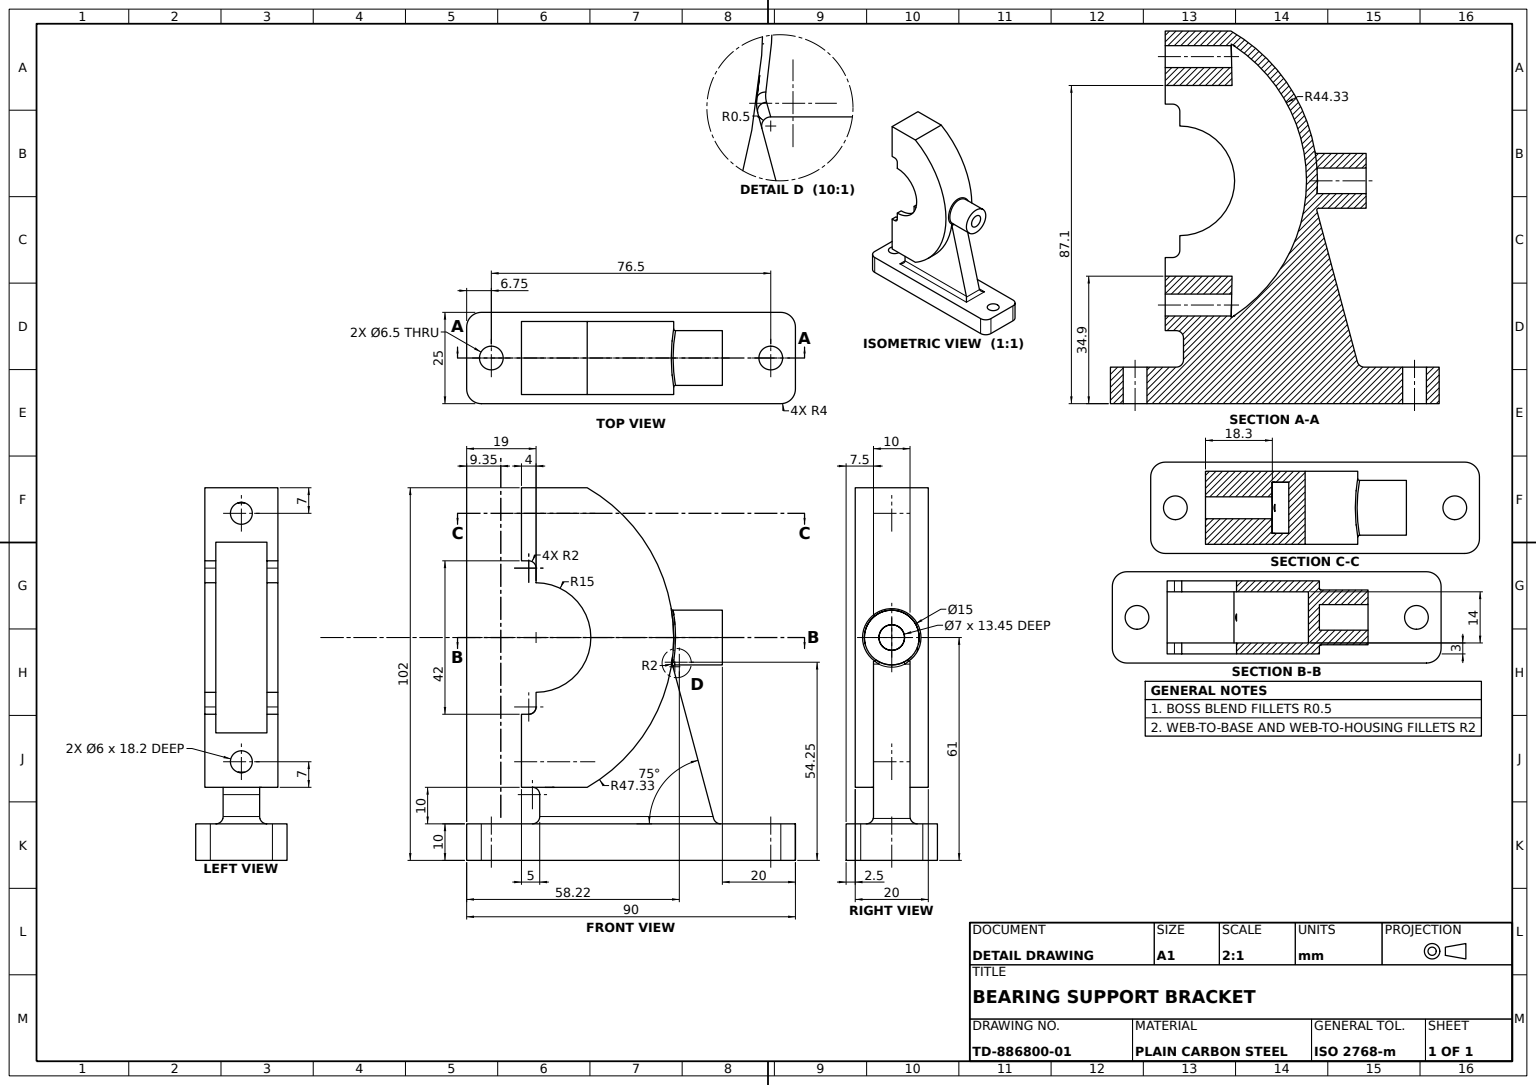
SolidWorks part; units mm, degrees
material "Plain Carbon Steel"
ref_plane "Front Plane" through (0, 0, 0) normal (0, 0, 1) x (1, 0, 0)
ref_plane "Top Plane" through (0, 0, 0) normal (0, 1, 0) x (1, 0, 0)
ref_plane "Right Plane" through (0, 0, 0) normal (1, 0, 0) x (0, 0, -1)
sketch "Base Plate Sketch" plane through (0, 0, 0) normal (0, 1, 0) x (1, 0, 0)
  line L1 (-41, 12.5) -> (41, 12.5)
  line L2 (-45, 8.5) -> (-45, -8.5)
  line L3 (-41, -12.5) -> (41, -12.5)
  line L4 (45, 8.5) -> (45, -8.5)
  line L5 (-45, 12.5) -> (45, -12.5) construction
  line L6 (-45, -12.5) -> (45, 12.5) construction
  arc A0 (41, -12.5) -> (45, -8.5) centre (41, -8.5) ccw
  arc A1 (41, 12.5) -> (45, 8.5) centre (41, 8.5) cw
  arc A2 (-45, -8.5) -> (-41, -12.5) centre (-41, -8.5) ccw
  arc A3 (-41, 12.5) -> (-45, 8.5) centre (-41, 8.5) ccw
  point P0 (0, 0)
  dimension "D3" = 4
  dimension "D1" = 90
  dimension "D2" = 25
extrude "Base Plate" add sketch "Base Plate Sketch" along normal blind 10
sketch "Mounting Holes Sketch" plane through (0, 10, 0) normal (0, 1, 0) x (1, 0, 0)
  line L0 (45, -8.5) -> (45, 8.5) construction
  line L1 (41, 12.5) -> (-41, 12.5) construction
  line L3 (-45, 8.5) -> (-45, -8.5) construction
  circle A0 centre (-38.25, 0) radius 3.25
  circle A1 centre (38.25, 0) radius 3.25
  dimension "D1" = 6.5
  dimension "D2" = 6.5
  dimension "D3" = 76.5
  dimension "D4" = 6.75
  dimension "D5" = 12.5
  dimension "D6" = 6.75
extrude "Mounting Holes 2xØ6.5" cut sketch "Mounting Holes Sketch" against normal blind 10
sketch "Upright Web Sketch" plane through (0, 10, 0) normal (0, 1, 0) x (1, 0, 0)
  line L1 (-24, 6) -> (24, 6)
  line L2 (-24, 6) -> (-24, -6)
  line L3 (-24, -6) -> (24, -6)
  line L4 (24, 6) -> (24, -6)
  line L5 (-24, 6) -> (24, -6) construction
  line L6 (-24, -6) -> (24, 6) construction
  point P0 (0, 0)
  dimension "D1" = 12
  dimension "D2" = 48
extrude "Upright Web" add sketch "Upright Web Sketch" along normal blind 30 draft 3
ref_plane "Plane1" through (0, 0, 10) normal (0, 0, 1) x (1, 0, 0)
sketch "Housing Half Sketch" plane through (0, 0, 10) normal (0, 0, 1) x (1, 0, 0)
  line L3 (-30, 82) -> (-26, 82)
  line L4 (-30, 102) -> (-12, 102)
  line L5 (-30, 102) -> (-12, 102)
  line L6 (-30, 20) -> (-12, 20)
  line L7 (-30, 40) -> (-30, 20)
  line L8 (-26, 82) -> (-26, 76)
  line L9 (-30, 102) -> (-30, 82)
  line L10 (-30, 40) -> (-26, 40)
  line L11 (-26, 40) -> (-26, 46)
  arc A0 (-12, 102) -> (-12, 20) centre (-35.6548, 61) cw
  arc A1 (-26, 76) -> (-26, 46) centre (-26, 61) cw
  dimension "D3" = 18
  dimension "D6" = 47.3344
  dimension "D14" = 15
  dimension "D1" = 82
  dimension "D2" = 20
  dimension "D4" = 18
  dimension "D5" = 102
  dimension "D7" = 4
  dimension "D8" = 6
  dimension "D9" = 20
  dimension "D10" = 4
  dimension "D11" = 6
  dimension "D12" = 48.4278
  dimension "D13" = 12
extrude "Housing Half" add sketch "Housing Half Sketch" against normal blind 3 separate body contours L8 A1 L11 L10 L7 L6 A0 L4 L9 L3
sketch "Housing Arc Cut Sketch" plane through (0, 0, 7) normal (0, 0, -1) x (-1, 0, 0)
  line L0 (12, 20) -> (30, 20)
  line L1 (30, 20) -> (30, 40)
  line L2 (30, 40) -> (-6.7663, 40)
  line L3 (-22.4278, 40) -> (22.4278, 40) construction
  line L4 (30, 102) -> (30, 82) construction
  arc A0 (-6.7663, 40) -> (12, 20) centre (35.6548, 61) ccw
  dimension "D1" = 47.3344
  dimension "D2" = 5.6548
  dimension "D3" = 18
extrude "Housing Arc Cut" cut sketch "Housing Arc Cut Sketch" along normal blind 20
sketch "Web Relief Cut Sketch" plane through (-24.4569, 1.2817, 0) normal (-0.9986, 0.0523, 0) x (0, 0, 1)
  line L0 (-5.4759, 18.744) -> (5.4759, 18.744) construction
  line L1 (6.1833, 18.8471) -> (-7.6646, 18.8471)
  line L2 (6.1833, 18.8471) -> (6.1833, 47.7969)
  line L3 (6.1833, 47.7969) -> (-7.6646, 47.7969)
  line L4 (-7.6646, 18.8471) -> (-7.6646, 47.7969)
  dimension "D1" = 0.7074
  dimension "D2" = 13.1405
  dimension "D3" = 0.1032
  dimension "D4" = 29.0529
extrude "Web Relief Cut" cut sketch "Web Relief Cut Sketch" against normal blind 60
sketch "Housing Lug Sketch" plane through (0, 0, 7) normal (0, 0, -1) x (-1, 0, 0)
  line L3 (30, 102) -> (12, 102)
  line L4 (12, 20) -> (30, 20)
  line L5 (12.8175, 23) -> (30, 23)
  line L6 (30, 99) -> (12.8175, 99)
  line L7 (12.8175, 23) -> (30, 23)
  line L8 (30, 99) -> (12.8175, 99)
  line L9 (30, 102) -> (30, 99)
  line L10 (30, 23) -> (30, 20)
  arc A3 (12, 102) -> (12, 20) centre (35.6548, 61) ccw
  arc A4 (12.8175, 99) -> (12.8175, 23) centre (35.6548, 61) ccw
  arc A5 (12.8175, 99) -> (12.8175, 23) centre (35.6548, 61) ccw
  dimension "D1" = 3
  dimension "D2" = 3
extrude "Housing Lug" add sketch "Housing Lug Sketch" along normal blind 14
sketch "Housing Flange Sketch" plane through (0, 0, -7) normal (0, 0, -1) x (-1, 0, 0)
  line L4 (30, 102) -> (30, 82)
  line L5 (30, 82) -> (26, 82)
  line L6 (30, 20) -> (12, 20)
  line L7 (12, 102) -> (30, 102)
  line L8 (30, 20) -> (12, 20)
  line L9 (12, 102) -> (30, 102)
  line L10 (26, 82) -> (26, 76)
  line L11 (26, 46) -> (26, 40)
  line L12 (26, 40) -> (30, 40)
  line L13 (30, 40) -> (30, 20)
  arc A5 (26, 76) -> (26, 46) centre (26, 61) ccw
  arc A6 (12, 102) -> (12, 20) centre (35.6548, 61) ccw
  arc A7 (12, 102) -> (12, 20) centre (35.6548, 61) ccw
  dimension "D2" = 15
  dimension "D1" = 3
extrude "Housing Flange" add sketch "Housing Flange Sketch" along normal blind 3
sketch "Housing Rib Sketch" plane through (0, 0, 10) normal (0, 0, 1) x (1, 0, 0)
  line L0 (-30, 102) -> (-30, 87.0998)
  line L1 (-30, 102) -> (-30, 82) construction
  line L2 (-30, 87.0998) -> (-11.7018, 87.0998)
  line L3 (-11.7018, 87.0998) -> (-12, 102)
  line L4 (-12, 102) -> (-30, 102)
  line L6 (-30, 20) -> (-30, 34.9)
  line L7 (-30, 40) -> (-30, 20) construction
  line L8 (-30, 34.9) -> (-11.7018, 34.9)
  line L9 (-11.7018, 34.9) -> (-12, 20)
  line L10 (-12, 20) -> (-30, 20)
  dimension "D1" = 14.9002
  dimension "D2" = 18.2982
  dimension "D3" = 14.9
  dimension "D4" = 23.5974
extrude "Housing Rib" add sketch "Housing Rib Sketch" against normal blind 20
sketch "Housing Relief Cut Sketch" plane through (0, 0.341, 6.5062) normal (0, 0.0523, 0.9986) x (1, 0, 0)
  line L0 (-23.4759, 19.686) -> (-24, 9.6723)
  line L3 (26.4801, 18.2381) -> (26.4801, 9.6723)
  line L4 (-12.0466, 19.686) -> (-24.6875, 19.686)
  line L5 (-24.6875, 19.686) -> (-24.6875, 9.6723)
  line L6 (-24.6875, 9.6723) -> (26.4801, 9.6723)
  line L7 (-12.0466, 19.686) -> (26.4801, 18.2381)
  line L8 (-23.4759, 19.686) -> (-21.5043, 19.686) construction
  line M5 (24, 9.6723) -> (23.5998, 17.319)
  line M6 (23.5998, 17.319) -> (-21.5043, 19.686)
  line M7 (-21.5043, 19.686) -> (-23.4759, 19.686)
  line M8 (-23.4759, 19.686) -> (-24, 9.6723)
  line M9 (-24, 9.6723) -> (24, 9.6723)
  dimension "D1" = 11.4293
  dimension "D2" = 49.956
  dimension "D3" = 1.2116
  dimension "D4" = 1.4479
extrude "Housing Relief Cut" cut sketch "Housing Relief Cut Sketch" against normal blind 15 contours M9 M5 M6 M7 M8 | L7 L4 L6 L3 M6 M5 | L5 L6 L4 M8
ref_plane "Plane2" through (0, 0, 5) normal (0, 0, 1) x (1, 0, 0)
sketch "Housing Body Sketch" plane through (0, 0, 5) normal (0, 0, 1) x (1, 0, 0)
  line L0 (-45, 10) -> (-45, 0) construction
  line L1 (-27, 20) -> (-12, 20)
  line L5 (-41, 10) -> (41, 10) construction
  line L6 (23, 10) -> (11.1774, 54.1226)
  line L7 (-25, 18) -> (-25, 9.9595)
  line L8 (-25, 9.9595) -> (23, 10)
  arc A0 (11.1774, 54.1226) -> (-12, 20) centre (-35.6548, 61) cw
  arc A1 (-25, 18) -> (-27, 20) centre (-27, 18) ccw
  dimension "D1" = 11.1774
  dimension "D2" = 2
  dimension "D3" = 47.3344
  dimension "D4" = 44.1226
  dimension "D5" = 15
  dimension "D6" = 8.0405
  dimension "D7" = 20
  dimension "D8" = 48
extrude "Housing Body" add sketch "Housing Body Sketch" against normal blind 10
sketch "Fill Block Sketch" plane through (0, 10, 0) normal (0, 1, 0) x (1, 0, 0)
  line L0 (-24.6875, 9.0206) -> (26.4801, 9.0206) construction
  line L1 (26.4801, -6) -> (-24.6875, -6)
  line L2 (26.4801, -6) -> (26.4801, 9.0206)
  line L3 (26.4801, 9.0206) -> (-24.6875, 9.0206)
  line L4 (-24.6875, -6) -> (-24.6875, 9.0206)
  line L5 (-25, -5) -> (-25, 5) construction
  dimension "D1" = 0.3125
extrude "Fill Block" add sketch "Fill Block Sketch" against normal blind 10
sketch "Bearing Seat Notch Sketch" plane through (0, 10, 0) normal (0, 1, 0) x (1, 0, 0)
  line L0 (-25, -5) -> (-25, 5) construction
  line L1 (-25, 5) -> (-4.0206, 5)
  line L2 (-25, 5) -> (-25, 11.478)
  line L3 (-25, 11.478) -> (-4.0206, 11.478)
  line L4 (-4.0206, 5) -> (-4.0206, 11.478)
  line L5 (-25, -5) -> (23, -5) construction
  dimension "D1" = 20.9794
  dimension "D2" = 16.478
extrude "Bearing Seat Notch" cut sketch "Bearing Seat Notch Sketch" along normal blind 10
fillet "Base To Housing Fillet R2" radius 2 4 edges at (-1, 10, -5) (-1, 10, 5) (23, 10, 0) (-25, 10, 0)
sketch "Split Bolt Holes Sketch" plane through (-30, 0, 0) normal (-1, 0, 0) x (0, 0, 1)
  line L0 (10, 102) -> (10, 82) construction
  line L1 (-10, 102) -> (10, 102) construction
  line L2 (-10, 20) -> (10, 20) construction
  line L3 (10, 40) -> (10, 20) construction
  circle A0 centre (0, 95) radius 3
  circle A1 centre (0, 27) radius 3
  dimension "D1" = 6
  dimension "D2" = 6
  dimension "D3" = 10
  dimension "D4" = 7
  dimension "D5" = 7
  dimension "D6" = 10
extrude "Split Bolt Holes" cut sketch "Split Bolt Holes Sketch" against normal blind 19
fillet "Flange Fillet R2" radius 2 4 edges at (-26, 82, -8.5) (-26, 82, 8.5) (-26, 40, 8.5) (-26, 40, -8.5)
fillet "Housing Edge Fillet R2" radius 2 1 edges at (11.1774, 54.1226, 0)
ref_plane "Plane3" through (25, 0, 0) normal (1, 0, 0) x (0, 0, -1)
sketch "Grease Nipple Boss Sketch" plane through (25, 0, 0) normal (1, 0, 0) x (0, 0, -1)
  line L0 (10, 102) -> (-10, 102) construction
  line L1 (10, 20) -> (10, 102) construction
  circle A0 centre (0, 61) radius 3.5
  circle A1 centre (0, 61) radius 7.5
  dimension "D1" = 15
  dimension "D2" = 7
  dimension "D3" = 41
  dimension "D4" = 10
extrude "Grease Nipple Boss" add sketch "Grease Nipple Boss Sketch" against normal blind 15
fillet "Grease Boss Fillet R0.5" radius 0.5 4 edges at (11.3442, 53.5, 0) (11.112, 53.6914, -1.6836)
